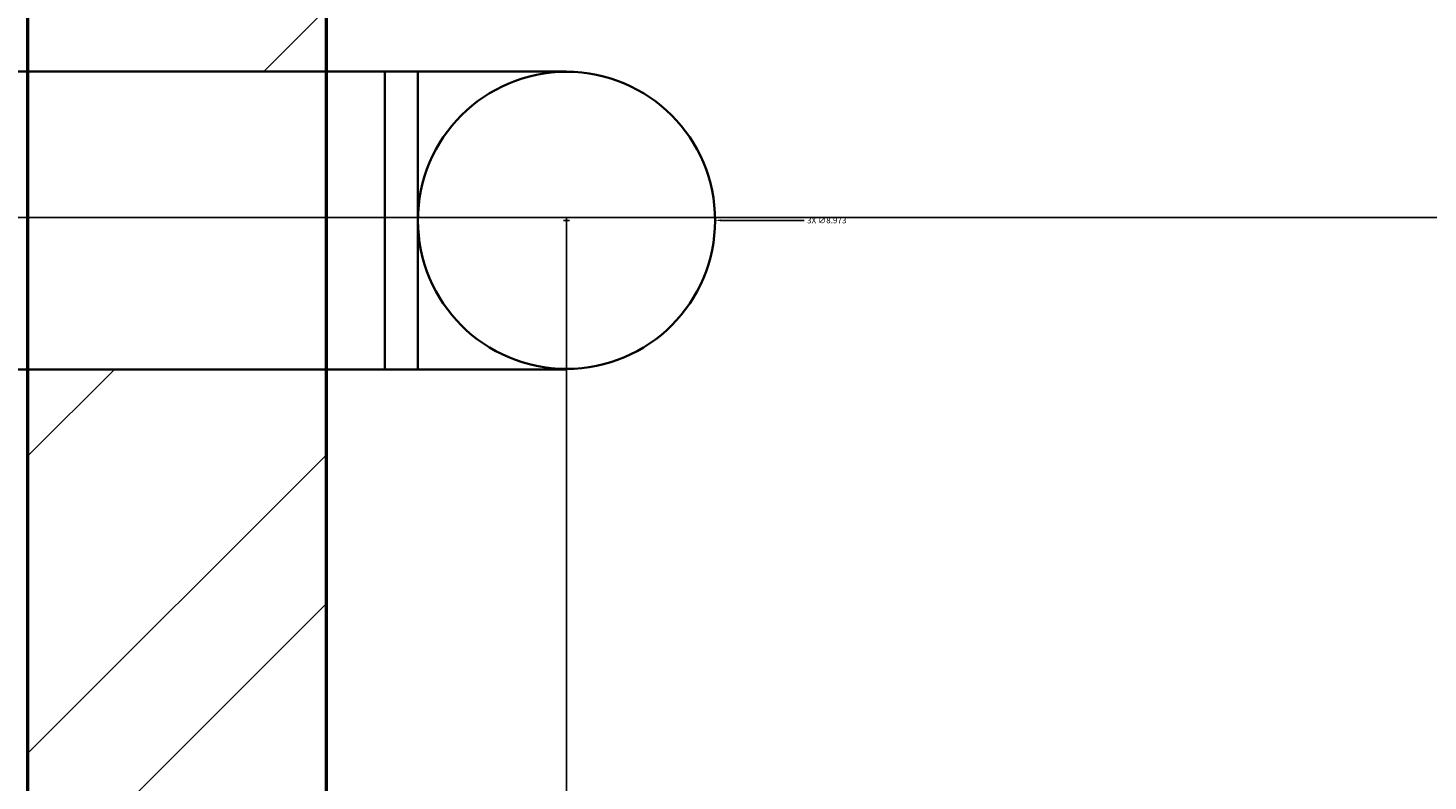
# Model space of a CAD drawing. Units: inches. Extents: x 2812 to 3051, y 1398 to 1659.
# Tile 47 of 65: x 2835 to 2878, y 1582 to 1605. Entities that reach past the tile are written whole.
import ezdxf

# ---------------------------------------------------------------- set-up
doc = ezdxf.new("R2010")
doc.units = ezdxf.units.IN
for name, color, linetype, lineweight in [('A-ANNO-DIMS', 2, 'Continuous', 18), ('P-SANR-PIPE', 4, 'Continuous', 35), ('S-CONC', 7, 'Continuous', 50), ('S-CONC-PATT', 8, 'Continuous', 18)]:
    doc.layers.add(name, color=color, linetype=linetype, lineweight=lineweight)
doc.styles.get("Standard").update_dxf_attribs({"font": 'arial.ttf'})
doc.dimstyles.get("Standard").update_dxf_attribs({"dimtxt": 0.18, "dimasz": 0.18, "dimexe": 0.18, "dimexo": 0.0625, "dimgap": 0.09, "dimtad": 0, "dimtih": 1, "dimtoh": 1, "dimdec": 4, "dimzin": 0, "dimdsep": 46, "dimtxsty": 'Standard', "dimcen": 0.09, "dimadec": 0, "dimazin": 0, "dimtfac": 1, "dimtdec": 4, "dimtofl": 0, "dimtmove": 0, "dimatfit": 3, "dimfxl": 1, "dimtolj": 1, "dimtzin": 0, "dimarcsym": 0})

# ---------------------------------------------------------------- blocks, each defined once
blk = doc.blocks.new('PIPE-BREAK')
for p, q in [((27.315, 9), (0.19, 9)), ((0.19, 0), (27.315, 0))]:
    blk.add_line(p, q)
blk.add_open_spline([(0.19, 0), (0.025, 1.41), (-0.305, 4.231), (1.347, 8.126), (0.19, 9)], degree=3)
blk = doc.blocks.new('*D28')
at = {"layer": 'A-ANNO-DIMS', "color": 0, "lineweight": -2, "transparency": 16777216}
for p, q in [((2851.646, 1598.667), (2851.646, 1397.505)), ((2844.385, 1559.757), (2844.385, 1397.505)), ((2844.565, 1397.685), (2847.64, 1397.685)), ((2851.466, 1397.685), (2848.391, 1397.685))]:
    blk.add_line(p, q, dxfattribs=at)
at = {"layer": 'A-ANNO-DIMS', "color": 0, "transparency": 16777216}
for points in [[(2844.565, 1397.715), (2844.565, 1397.655), (2844.385, 1397.685)], [(2851.466, 1397.715), (2851.466, 1397.655), (2851.646, 1397.685)]]:
    blk.add_solid(points, dxfattribs=at)
at = {"layer": 'Defpoints', "color": 0, "transparency": 16777216}
for p in [(2851.646, 1598.73), (2844.385, 1559.82), (2851.646, 1397.685)]:
    blk.add_point(p, dxfattribs=at)
at = {"layer": 'A-ANNO-DIMS', "color": 0, "transparency": 16777216, "insert": (2848.016, 1397.685), "char_height": 0.18, "attachment_point": 5}
blk.add_mtext('\\A1;7.261', dxfattribs=at)
blk = doc.blocks.new('*D37')
at = {"layer": 'A-ANNO-DIMS', "color": 0, "lineweight": -2, "transparency": 16777216}
for p, q in [((2910.679, 1598.82), (2811.806, 1598.82)), ((2811.986, 1598.64), (2811.986, 1579.502)), ((2811.986, 1560), (2811.986, 1579.138)), ((2883.322, 1559.82), (2811.806, 1559.82))]:
    blk.add_line(p, q, dxfattribs=at)
at = {"layer": 'A-ANNO-DIMS', "color": 0, "transparency": 16777216}
for points in [[(2811.956, 1598.64), (2812.016, 1598.64), (2811.986, 1598.82)], [(2811.956, 1560), (2812.016, 1560), (2811.986, 1559.82)]]:
    blk.add_solid(points, dxfattribs=at)
at = {"layer": 'Defpoints', "color": 0, "transparency": 16777216}
for p in [(2811.986, 1598.82), (2910.742, 1598.82), (2883.385, 1559.82)]:
    blk.add_point(p, dxfattribs=at)
at = {"layer": 'A-ANNO-DIMS', "color": 0, "transparency": 16777216, "insert": (2811.986, 1579.32), "char_height": 0.18, "attachment_point": 5}
blk.add_mtext('\\A1;39', dxfattribs=at)
blk = doc.blocks.new('*D38')
at = {"layer": 'A-ANNO-DIMS', "color": 0, "lineweight": -2, "transparency": 16777216}
for p, q in [((2896.322, 1625.82), (2811.806, 1625.82)), ((2811.986, 1625.64), (2811.986, 1612.5)), ((2811.986, 1599), (2811.986, 1612.14)), ((2910.679, 1598.82), (2811.806, 1598.82))]:
    blk.add_line(p, q, dxfattribs=at)
at = {"layer": 'A-ANNO-DIMS', "color": 0, "transparency": 16777216}
for points in [[(2811.956, 1625.64), (2812.016, 1625.64), (2811.986, 1625.82)], [(2811.956, 1599), (2812.016, 1599), (2811.986, 1598.82)]]:
    blk.add_solid(points, dxfattribs=at)
at = {"layer": 'Defpoints', "color": 0, "transparency": 16777216}
for p in [(2811.986, 1625.82), (2896.385, 1625.82), (2910.742, 1598.82)]:
    blk.add_point(p, dxfattribs=at)
at = {"layer": 'A-ANNO-DIMS', "color": 0, "transparency": 16777216, "insert": (2811.986, 1612.32), "char_height": 0.18, "attachment_point": 5}
blk.add_mtext('\\A1;27', dxfattribs=at)
blk = doc.blocks.new('*D85')
at = {"layer": 'A-ANNO-DIMS', "color": 0, "lineweight": -2, "transparency": 16777216}
for p, q in [((2851.556, 1598.73), (2851.736, 1598.73)), ((2851.646, 1598.64), (2851.646, 1598.82)), ((2858.825, 1598.73), (2856.313, 1598.73))]:
    blk.add_line(p, q, dxfattribs=at)
at = {"layer": 'A-ANNO-DIMS', "color": 0, "transparency": 16777216}
blk.add_solid([(2856.313, 1598.76), (2856.313, 1598.7), (2856.133, 1598.73)], dxfattribs=at)
at = {"layer": 'Defpoints', "color": 0, "transparency": 16777216}
for p in [(2847.16, 1598.729), (2856.133, 1598.73)]:
    blk.add_point(p, dxfattribs=at)
at = {"layer": 'A-ANNO-DIMS', "color": 0, "transparency": 16777216, "insert": (2859.505, 1598.73), "char_height": 0.18, "attachment_point": 5}
blk.add_mtext('\\A1;3X ∅8.973', dxfattribs=at)

msp = doc.modelspace()

# ---------------------------------------------------------------- hatches: boundary and pattern name
at = {"layer": 'S-CONC-PATT'}
h = msp.add_hatch(dxfattribs=at)
h.set_pattern_fill('ANSI32', color=256)
h.paths.add_polyline_path([(3027.3849, 1646.82), (2835.3849, 1646.82), (2835.3849, 1603.2296), (2844.3849, 1603.2296), (2844.3849, 1637.82), (3018.3849, 1637.82), (3018.3849, 1602.5441), (3027.3849, 1602.5441)])
h.paths.add_polyline_path([(2844.3849, 1594.2296), (2835.3849, 1594.2296), (2835.3849, 1550.82), (3027.3849, 1550.82), (3027.3849, 1593.5441), (3018.3849, 1593.5441), (3018.3849, 1559.82), (2844.3849, 1559.82)])
h.paths.add_polyline_path([(2844.3849, 1482.0354), (2835.3849, 1482.0354), (2835.3849, 1463.4959), (2844.3849, 1463.4959)])
h.paths.add_polyline_path([(2844.3849, 1461.4959), (2835.3849, 1461.4959), (2835.3849, 1416.0354), (2844.3849, 1416.0354)])
h.paths.add_polyline_path([(3027.3849, 1482.0354), (3018.3849, 1482.0354), (3018.3849, 1463.2854), (3027.3849, 1463.2854)])
h.paths.add_polyline_path([(3027.3849, 1461.2854), (3018.3849, 1461.2854), (3018.3849, 1416.0354), (3027.3849, 1416.0354)])
h.paths.add_polyline_path([(2961.3849, 1448.4738), (2952.3849, 1448.4738), (2952.3849, 1416.0354), (2961.3849, 1416.0354)])
h.paths.add_polyline_path([(2961.3849, 1462.3026), (2952.3849, 1462.3026), (2952.3849, 1450.4738), (2961.3849, 1450.4738)])
h.paths.add_polyline_path([(2961.3849, 1472.0354), (2952.3849, 1472.0354), (2952.3849, 1462.3026), (2961.3849, 1462.3026)])

# ---------------------------------------------------------------- linework, layer by layer
at = {"layer": 'P-SANR-PIPE'}
for p, q in [((2846.1595, 1603.2296), (2846.1595, 1594.2296)), ((2847.1595, 1594.2296), (2847.1595, 1603.2296))]:
    msp.add_line(p, q, dxfattribs=at)
msp.add_circle((2851.6462, 1598.7296), 4.4867, dxfattribs=at)
at = {"layer": 'S-CONC'}
for p, q in [((2835.3849, 1550.82), (2835.3849, 1646.82)), ((2844.3849, 1637.82), (2844.3849, 1559.82))]:
    msp.add_line(p, q, dxfattribs=at)

# ---------------------------------------------------------------- block references
at = {"layer": 'P-SANR-PIPE'}
msp.add_blockref('PIPE-BREAK', (2824.331, 1594.23), dxfattribs=at)

# ---------------------------------------------------------------- dimensions: what is measured, and where the dimension line sits
at = {"layer": 'A-ANNO-DIMS'}
for base, p1, p2, picture, middle in [((2811.9855, 1625.82), (2910.7415, 1598.82), (2896.3849, 1625.82), '*D38', (2811.9855, 1612.32)), ((2811.9855, 1598.82), (2883.3849, 1559.82), (2910.7415, 1598.82), '*D37', (2811.9855, 1579.32))]:
    dim = msp.add_linear_dim(base=base, p1=p1, p2=p2, angle=90, dimstyle='Standard', override={"dimdec": 0, "dimlfac": 1, "dimrnd": 0, "dimzin": 0, "dimdsep": 46, "dimlunit": 2}, dxfattribs=at)
    dim.commit()
    dim.dimension.update_dxf_attribs({"geometry": picture, "text_midpoint": middle})
dim = msp.add_diameter_dim_2p(p1=(2847.1595, 1598.7293), p2=(2856.1329, 1598.73), text='3X <>', dimstyle='Standard', override={"dimdec": 3, "dimlfac": 1, "dimrnd": 0, "dimzin": 0, "dimdsep": 46, "dimlunit": 2}, dxfattribs=at)
dim.commit()
dim.dimension.update_dxf_attribs({"geometry": '*D85', "text_midpoint": (2858.8249, 1598.7302), "dimtype": 163})
dim = msp.add_linear_dim(base=(2851.6462, 1397.6854), p1=(2844.3849, 1559.82), p2=(2851.6462, 1598.7296), dimstyle='Standard', override={"dimdec": 3, "dimlfac": 1, "dimrnd": 0, "dimzin": 0, "dimdsep": 46, "dimlunit": 2}, dxfattribs=at)
dim.commit()
dim.dimension.update_dxf_attribs({"geometry": '*D28', "text_midpoint": (2848.0156, 1397.6854)})

doc.saveas('drawing.dxf')
